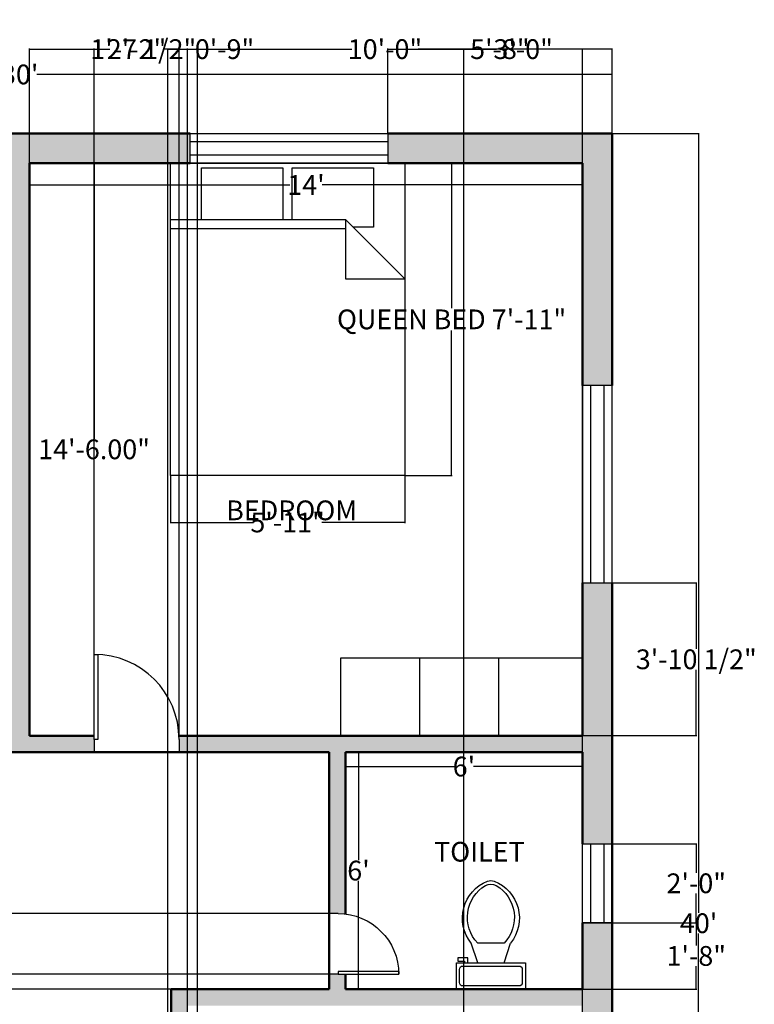
# Model space of a CAD drawing. Units: inches. Extents: x -19 to 426, y -15 to 535.
# Tile 4 of 4: x 202 to 426, y 235 to 535. Entities that reach past the tile are written whole.
import ezdxf

# ---------------------------------------------------------------- set-up
doc = ezdxf.new("R2010")
doc.units = ezdxf.units.IN
doc.header["$MEASUREMENT"] = 0
for name, color, linetype, lineweight in [('A-ANNO-DIMS', 3, 'Continuous', 18), ('A-AREA-IDEN', 7, 'Continuous', 25), ('A-DOOR', 4, 'Continuous', 25), ('A-FLOR-CABN', 40, 'Continuous', 25), ('A-FLOR-FIXT', 8, 'Continuous', 25), ('A-FURN', 40, 'Continuous', 25), ('A-GLAZ', 40, 'Continuous', 25), ('A-WALL', 7, 'Continuous', 50), ('A-WALL-PATT', 5, 'Continuous', 13)]:
    doc.layers.add(name, color=color, linetype=linetype, lineweight=lineweight)
doc.styles.get("Standard").update_dxf_attribs({"font": 'arial.ttf'})
doc.dimstyles.get("Standard").update_dxf_attribs({"dimtxt": 6, "dimasz": 0.18, "dimexe": 0.18, "dimexo": 0.0625, "dimgap": 0.09, "dimtad": 0, "dimtih": 1, "dimtoh": 1, "dimzin": 0, "dimdsep": 46, "dimlunit": 3, "dimtxsty": 'Standard', "dimcen": 0.09, "dimadec": 0, "dimazin": 0, "dimtfac": 1, "dimtofl": 0, "dimtmove": 0, "dimatfit": 3, "dimfxl": 1, "dimtolj": 1, "dimtzin": 0, "dimarcsym": 0})

# ---------------------------------------------------------------- blocks, each defined once
blk = doc.blocks.new('*D2')
at = {"layer": 'A-ANNO-DIMS', "color": 0, "lineweight": -2, "transparency": 16777216}
for p, q in [((301.43, 311.94), (301.43, 307.44)), ((373.43, 311.94), (373.43, 307.44)), ((301.61, 307.62), (334.57, 307.62)), ((373.25, 307.62), (340.3, 307.62))]:
    blk.add_line(p, q, dxfattribs=at)
at = {"layer": 'A-ANNO-DIMS', "color": 0, "transparency": 16777216}
for points in [[(301.61, 307.65), (301.61, 307.59), (301.43, 307.62)], [(373.25, 307.65), (373.25, 307.59), (373.43, 307.62)]]:
    blk.add_solid(points, dxfattribs=at)
at = {"layer": 'Defpoints', "color": 0, "transparency": 16777216}
for p in [(301.43, 312.01), (373.43, 312.01), (373.43, 307.62)]:
    blk.add_point(p, dxfattribs=at)
at = {"layer": 'A-ANNO-DIMS', "color": 0, "transparency": 16777216, "insert": (337.43, 307.62), "char_height": 6, "attachment_point": 5}
blk.add_mtext("\\A1;6'", dxfattribs=at)
blk = doc.blocks.new('*D3')
at = {"layer": 'A-ANNO-DIMS', "color": 0, "lineweight": -2, "transparency": 16777216}
for p, q in [((301.49, 312.01), (305.56, 312.01)), ((305.38, 311.83), (305.38, 279.16)), ((305.38, 240.19), (305.38, 272.85)), ((301.49, 240.01), (305.56, 240.01))]:
    blk.add_line(p, q, dxfattribs=at)
at = {"layer": 'A-ANNO-DIMS', "color": 0, "transparency": 16777216}
for points in [[(305.35, 311.83), (305.41, 311.83), (305.38, 312.01)], [(305.35, 240.19), (305.41, 240.19), (305.38, 240.01)]]:
    blk.add_solid(points, dxfattribs=at)
at = {"layer": 'Defpoints', "color": 0, "transparency": 16777216}
for p in [(301.43, 312.01), (301.43, 240.01), (305.38, 240.01)]:
    blk.add_point(p, dxfattribs=at)
at = {"layer": 'A-ANNO-DIMS', "color": 0, "transparency": 16777216, "insert": (305.38, 276.01), "char_height": 6, "attachment_point": 5}
blk.add_mtext("\\A1;6'", dxfattribs=at)
blk = doc.blocks.new('*D4')
at = {"layer": 'A-ANNO-DIMS', "color": 0, "lineweight": -2, "transparency": 16777216}
for p, q in [((205.43, 490.94), (205.43, 484.15)), ((373.43, 490.94), (373.43, 484.15)), ((205.61, 484.33), (284.53, 484.33)), ((373.25, 484.33), (294.33, 484.33))]:
    blk.add_line(p, q, dxfattribs=at)
at = {"layer": 'A-ANNO-DIMS', "color": 0, "transparency": 16777216}
for points in [[(205.61, 484.36), (205.61, 484.3), (205.43, 484.33)], [(373.25, 484.36), (373.25, 484.3), (373.43, 484.33)]]:
    blk.add_solid(points, dxfattribs=at)
at = {"layer": 'Defpoints', "color": 0, "transparency": 16777216}
for p in [(205.43, 491.01), (373.43, 491.01), (373.43, 484.33)]:
    blk.add_point(p, dxfattribs=at)
at = {"layer": 'A-ANNO-DIMS', "color": 0, "transparency": 16777216, "insert": (289.43, 484.33), "char_height": 6, "attachment_point": 5}
blk.add_mtext("\\A1;14'", dxfattribs=at)
blk = doc.blocks.new('Bed - Queen')
for p, q in [((0, -80.00003), (0, 0)), ((0, 0), (59.99999, 0)), ((59.99999, 0), (59.99999, -80.00003)), ((7.99999, -1.2), (28.79998, -1.2)), ((7.99999, -14.4), (7.99999, -1.2)), ((28.79998, -1.2), (28.79998, -14.4)), ((31.19999, -1.2), (51.99999, -1.2)), ((31.19999, -14.4), (31.19999, -1.2)), ((51.99999, -1.2), (51.99999, -16.4)), ((0, -14.4), (44.8, -14.4)), ((59.99999, -29.6), (44.8, -14.4)), ((44.8, -14.4), (44.8, -29.6)), ((44.8, -16.8), (0, -16.8)), ((51.99999, -16.4), (46.79936, -16.4)), ((44.8, -29.6), (59.99999, -29.6)), ((59.99999, -80.00003), (0, -80.00003))]:
    blk.add_line(p, q)
blk = doc.blocks.new('*U9')
for p, q in [((0, 0), (0, -6)), ((40, 0), (40, -6))]:
    blk.add_line(p, q)
blk.add_lwpolyline([(0, 0), (0, 40), (1.75, 40), (1.75, 0)], close=True)
blk.add_arc((0, 0), 40, 0, 90)
blk = doc.blocks.new('*U7')
for p, q in [((9.5, -6), (9.5, -2)), ((-10, -8.5), (-8, -8.5)), ((-10, -9.5), (-10, -8.5)), ((-8, -8.5), (-8, -8)), ((-7, -8), (-7, -9.5)), ((-4, -8), (-6, -14)), ((4, -8), (6, -14)), ((-7, -9.5), (-10, -9.5)), ((4, -14), (-4, -14))]:
    blk.add_line(p, q)
blk.add_lwpolyline([(10.5, -8), (10.5, 0), (-10.5, 0), (-10.5, -8)], close=True)
for points in [[(-9.5, -2), (-9.5, -6)], [(8.5, -1), (-8.5, -1)], [(-8.5, -7), (8.5, -7)]]:
    blk.add_lwpolyline(points)
for centre, radius, start, end in [((-8.62, -1.88), 0.884, 81.8699, 188.1301), ((8.62, -1.88), 0.884, 351.8699, 98.1301), ((-8.62, -6.12), 0.884, 171.8699, 278.1301), ((8.62, -6.12), 0.884, 261.8699, 8.1301), ((3.52, -21.58), 12.17, 141.4691, 247.9714), ((4.2, -21.82), 11.33, 136.3677, 238.9468), ((-3.52, -21.58), 12.17, 292.0284, 38.5307), ((-4.2, -21.82), 11.33, 301.053, 43.6321), ((0, -27.88), 4, 245.7318, 294.2682), ((0, -29), 4, 254.8605, 285.1395)]:
    blk.add_arc(centre, radius, start, end)
blk = doc.blocks.new('*D15')
at = {"layer": 'A-ANNO-DIMS', "color": 0, "lineweight": -2, "transparency": 16777216}
for p, q in [((205.49, 491.01), (225.21, 491.01)), ((225.03, 490.83), (225.03, 407.16)), ((225.03, 317.19), (225.03, 400.85)), ((205.49, 317.01), (225.21, 317.01))]:
    blk.add_line(p, q, dxfattribs=at)
at = {"layer": 'A-ANNO-DIMS', "color": 0, "transparency": 16777216}
for points in [[(225, 490.83), (225.06, 490.83), (225.03, 491.01)], [(225, 317.19), (225.06, 317.19), (225.03, 317.01)]]:
    blk.add_solid(points, dxfattribs=at)
at = {"layer": 'Defpoints', "color": 0, "transparency": 16777216}
for p in [(205.43, 491.01), (205.43, 317.01), (225.03, 317.01)]:
    blk.add_point(p, dxfattribs=at)
at = {"layer": 'A-ANNO-DIMS', "color": 0, "transparency": 16777216, "insert": (225.03, 404.01), "char_height": 6, "attachment_point": 5}
blk.add_mtext('\\A1;14\'-6.00"', dxfattribs=at)
blk = doc.blocks.new('*D18')
at = {"layer": 'A-ANNO-DIMS', "color": 0, "lineweight": -2, "transparency": 16777216}
for p, q in [((22.43, 500.07), (22.43, 518.1)), ((22.61, 517.92), (197.25, 517.92)), ((382.25, 517.92), (207.61, 517.92)), ((382.43, 500.07), (382.43, 518.1))]:
    blk.add_line(p, q, dxfattribs=at)
at = {"layer": 'A-ANNO-DIMS', "color": 0, "transparency": 16777216}
for points in [[(22.61, 517.95), (22.61, 517.89), (22.43, 517.92)], [(382.25, 517.95), (382.25, 517.89), (382.43, 517.92)]]:
    blk.add_solid(points, dxfattribs=at)
at = {"layer": 'Defpoints', "color": 0, "transparency": 16777216}
for p in [(382.43, 517.92), (22.43, 500.01), (382.43, 500.01)]:
    blk.add_point(p, dxfattribs=at)
at = {"layer": 'A-ANNO-DIMS', "color": 0, "transparency": 16777216, "insert": (202.43, 517.92), "char_height": 6, "attachment_point": 5}
blk.add_mtext("\\A1;30'", dxfattribs=at)
blk = doc.blocks.new('*D19')
at = {"layer": 'A-ANNO-DIMS', "color": 0, "lineweight": -2, "transparency": 16777216}
for p, q in [((382.49, 500.01), (408.92, 500.01)), ((408.74, 499.83), (408.74, 263.16)), ((408.74, 20.19), (408.74, 256.85)), ((382.49, 20.01), (408.92, 20.01))]:
    blk.add_line(p, q, dxfattribs=at)
at = {"layer": 'A-ANNO-DIMS', "color": 0, "transparency": 16777216}
for points in [[(408.71, 499.83), (408.77, 499.83), (408.74, 500.01)], [(408.71, 20.19), (408.77, 20.19), (408.74, 20.01)]]:
    blk.add_solid(points, dxfattribs=at)
at = {"layer": 'Defpoints', "color": 0, "transparency": 16777216}
for p in [(382.43, 500.01), (382.43, 20.01), (408.74, 20.01)]:
    blk.add_point(p, dxfattribs=at)
at = {"layer": 'A-ANNO-DIMS', "color": 0, "transparency": 16777216, "insert": (408.74, 260.01), "char_height": 6, "attachment_point": 5}
blk.add_mtext("\\A1;40'", dxfattribs=at)
blk = doc.blocks.new('WIN-60IN')
for p, q in [((0, 6.5), (60, 6.5)), ((0, 2.5), (60, 2.5))]:
    blk.add_line(p, q)
blk.add_lwpolyline([(0, 9), (60, 9), (60, 0), (0, 0)], close=True)
blk = doc.blocks.new('*D24')
at = {"layer": 'A-ANNO-DIMS', "color": 0, "lineweight": -2, "transparency": 16777216}
for p, q in [((319.5, 490.97), (333.86, 490.97)), ((333.68, 490.79), (333.68, 446.87)), ((333.68, 396.21), (333.68, 440.12)), ((319.5, 396.03), (333.86, 396.03))]:
    blk.add_line(p, q, dxfattribs=at)
at = {"layer": 'A-ANNO-DIMS', "color": 0, "transparency": 16777216}
for points in [[(333.65, 490.79), (333.71, 490.79), (333.68, 490.97)], [(333.65, 396.21), (333.71, 396.21), (333.68, 396.03)]]:
    blk.add_solid(points, dxfattribs=at)
at = {"layer": 'Defpoints', "color": 0, "transparency": 16777216}
for p in [(319.44, 490.97), (333.68, 490.97), (319.44, 396.03)]:
    blk.add_point(p, dxfattribs=at)
at = {"layer": 'A-ANNO-DIMS', "color": 0, "transparency": 16777216, "insert": (333.68, 443.5), "char_height": 6, "attachment_point": 5}
blk.add_mtext('\\A1;QUEEN BED 7\'-11"', dxfattribs=at)
blk = doc.blocks.new('*D25')
at = {"layer": 'A-ANNO-DIMS', "color": 0, "lineweight": -2, "transparency": 16777216}
for p, q in [((248.23, 395.97), (248.23, 381.61)), ((319.44, 395.97), (319.44, 381.61)), ((248.41, 381.79), (273.44, 381.79)), ((319.26, 381.79), (294.23, 381.79))]:
    blk.add_line(p, q, dxfattribs=at)
at = {"layer": 'A-ANNO-DIMS', "color": 0, "transparency": 16777216}
for points in [[(248.41, 381.82), (248.41, 381.76), (248.23, 381.79)], [(319.26, 381.82), (319.26, 381.76), (319.44, 381.79)]]:
    blk.add_solid(points, dxfattribs=at)
at = {"layer": 'Defpoints', "color": 0, "transparency": 16777216}
for p in [(248.23, 396.03), (319.44, 396.03), (319.44, 381.79)]:
    blk.add_point(p, dxfattribs=at)
at = {"layer": 'A-ANNO-DIMS', "color": 0, "transparency": 16777216, "insert": (283.84, 381.79), "char_height": 6, "attachment_point": 5}
blk.add_mtext('\\A1;5\'-11"', dxfattribs=at)
blk = doc.blocks.new('*D32')
at = {"layer": 'A-ANNO-DIMS', "color": 0, "lineweight": -2, "transparency": 16777216}
for p, q in [((253.43, 115.07), (253.43, 525.79)), ((253.61, 525.61), (303.32, 525.61)), ((373.25, 525.61), (323.55, 525.61)), ((373.43, 115.07), (373.43, 525.79))]:
    blk.add_line(p, q, dxfattribs=at)
at = {"layer": 'A-ANNO-DIMS', "color": 0, "transparency": 16777216}
for points in [[(253.61, 525.64), (253.61, 525.58), (253.43, 525.61)], [(373.25, 525.64), (373.25, 525.58), (373.43, 525.61)]]:
    blk.add_solid(points, dxfattribs=at)
at = {"layer": 'Defpoints', "color": 0, "transparency": 16777216}
for p in [(373.43, 525.61), (253.43, 115.01), (373.43, 115.01)]:
    blk.add_point(p, dxfattribs=at)
at = {"layer": 'A-ANNO-DIMS', "color": 0, "transparency": 16777216, "insert": (313.43, 525.61), "char_height": 6, "attachment_point": 5}
blk.add_mtext('\\A1;10\'-0"', dxfattribs=at)
blk = doc.blocks.new('*D37')
at = {"layer": 'A-ANNO-DIMS', "color": 0, "lineweight": -2, "transparency": 16777216}
for p, q in [((314.27, 500.07), (314.27, 525.79)), ((314.45, 525.61), (340.29, 525.61)), ((382.25, 525.61), (356.42, 525.61)), ((382.43, 500.07), (382.43, 525.79))]:
    blk.add_line(p, q, dxfattribs=at)
at = {"layer": 'A-ANNO-DIMS', "color": 0, "transparency": 16777216}
for points in [[(314.45, 525.64), (314.45, 525.58), (314.27, 525.61)], [(382.25, 525.64), (382.25, 525.58), (382.43, 525.61)]]:
    blk.add_solid(points, dxfattribs=at)
at = {"layer": 'Defpoints', "color": 0, "transparency": 16777216}
for p in [(382.43, 525.61), (314.27, 500.01), (382.43, 500.01)]:
    blk.add_point(p, dxfattribs=at)
at = {"layer": 'A-ANNO-DIMS', "color": 0, "transparency": 16777216, "insert": (348.35, 525.61), "char_height": 6, "attachment_point": 5}
blk.add_mtext('\\A1;5\'-8"', dxfattribs=at)
blk = doc.blocks.new('*D48')
at = {"layer": 'A-ANNO-DIMS', "color": 0, "lineweight": -2, "transparency": 16777216}
for p, q in [((373.49, 260.15), (408.21, 260.15)), ((408.03, 259.97), (408.03, 253.23)), ((408.03, 240.19), (408.03, 246.93)), ((373.49, 240.01), (408.21, 240.01))]:
    blk.add_line(p, q, dxfattribs=at)
at = {"layer": 'A-ANNO-DIMS', "color": 0, "transparency": 16777216}
for points in [[(408, 259.97), (408.06, 259.97), (408.03, 260.15)], [(408, 240.19), (408.06, 240.19), (408.03, 240.01)]]:
    blk.add_solid(points, dxfattribs=at)
at = {"layer": 'Defpoints', "color": 0, "transparency": 16777216}
for p in [(373.43, 260.15), (408.03, 260.15), (373.43, 240.01)]:
    blk.add_point(p, dxfattribs=at)
at = {"layer": 'A-ANNO-DIMS', "color": 0, "transparency": 16777216, "insert": (408.03, 250.08), "char_height": 6, "attachment_point": 5}
blk.add_mtext('\\A1;1\'-8"', dxfattribs=at)
blk = doc.blocks.new('*D49')
at = {"layer": 'A-ANNO-DIMS', "color": 0, "lineweight": -2, "transparency": 16777216}
for p, q in [((373.49, 284.15), (408.21, 284.15)), ((408.03, 283.97), (408.03, 275.3)), ((408.03, 260.33), (408.03, 269)), ((373.49, 260.15), (408.21, 260.15))]:
    blk.add_line(p, q, dxfattribs=at)
at = {"layer": 'A-ANNO-DIMS', "color": 0, "transparency": 16777216}
for points in [[(408, 283.97), (408.06, 283.97), (408.03, 284.15)], [(408, 260.33), (408.06, 260.33), (408.03, 260.15)]]:
    blk.add_solid(points, dxfattribs=at)
at = {"layer": 'Defpoints', "color": 0, "transparency": 16777216}
for p in [(373.43, 284.15), (408.03, 284.15), (373.43, 260.15)]:
    blk.add_point(p, dxfattribs=at)
at = {"layer": 'A-ANNO-DIMS', "color": 0, "transparency": 16777216, "insert": (408.03, 272.15), "char_height": 6, "attachment_point": 5}
blk.add_mtext('\\A1;2\'-0"', dxfattribs=at)
blk = doc.blocks.new('*D50')
at = {"layer": 'A-ANNO-DIMS', "color": 0, "lineweight": -2, "transparency": 16777216}
for p, q in [((373.49, 363.41), (408.21, 363.41)), ((408.03, 363.23), (408.03, 343.4)), ((408.03, 317.19), (408.03, 337.01)), ((373.49, 317.01), (408.21, 317.01))]:
    blk.add_line(p, q, dxfattribs=at)
at = {"layer": 'A-ANNO-DIMS', "color": 0, "transparency": 16777216}
for points in [[(408, 363.23), (408.06, 363.23), (408.03, 363.41)], [(408, 317.19), (408.06, 317.19), (408.03, 317.01)]]:
    blk.add_solid(points, dxfattribs=at)
at = {"layer": 'Defpoints', "color": 0, "transparency": 16777216}
for p in [(373.43, 363.41), (408.03, 363.41), (373.43, 317.01)]:
    blk.add_point(p, dxfattribs=at)
at = {"layer": 'A-ANNO-DIMS', "color": 0, "transparency": 16777216, "insert": (408.03, 340.21), "char_height": 6, "attachment_point": 5}
blk.add_mtext('\\A1;3\'-10 1/2"', dxfattribs=at)
blk = doc.blocks.new('*D53')
at = {"layer": 'A-ANNO-DIMS', "color": 0, "lineweight": -2, "transparency": 16777216}
for p, q in [((205.43, 317.07), (205.43, 525.79)), ((205.61, 525.61), (224.85, 525.61)), ((225.03, 317.07), (225.03, 525.79)), ((225.03, 525.61), (225.21, 525.61))]:
    blk.add_line(p, q, dxfattribs=at)
at = {"layer": 'A-ANNO-DIMS', "color": 0, "transparency": 16777216}
for points in [[(205.61, 525.64), (205.61, 525.58), (205.43, 525.61)], [(224.85, 525.64), (224.85, 525.58), (225.03, 525.61)]]:
    blk.add_solid(points, dxfattribs=at)
at = {"layer": 'Defpoints', "color": 0, "transparency": 16777216}
for p in [(225.03, 525.61), (205.43, 317.01), (225.03, 317.01)]:
    blk.add_point(p, dxfattribs=at)
at = {"layer": 'A-ANNO-DIMS', "color": 0, "transparency": 16777216, "insert": (239.99, 525.61), "char_height": 6, "attachment_point": 5}
blk.add_mtext('\\A1;1\'-7 1/2"', dxfattribs=at)
blk = doc.blocks.new('*D54')
at = {"layer": 'A-ANNO-DIMS', "color": 0, "lineweight": -2, "transparency": 16777216}
for p, q in [((225.03, 317.07), (225.03, 525.79)), ((225.21, 525.61), (229.82, 525.61)), ((250.67, 525.61), (246.06, 525.61)), ((250.85, 317.07), (250.85, 525.79))]:
    blk.add_line(p, q, dxfattribs=at)
at = {"layer": 'A-ANNO-DIMS', "color": 0, "transparency": 16777216}
for points in [[(225.21, 525.64), (225.21, 525.58), (225.03, 525.61)], [(250.67, 525.64), (250.67, 525.58), (250.85, 525.61)]]:
    blk.add_solid(points, dxfattribs=at)
at = {"layer": 'Defpoints', "color": 0, "transparency": 16777216}
for p in [(250.85, 525.61), (225.03, 317.01), (250.85, 317.01)]:
    blk.add_point(p, dxfattribs=at)
at = {"layer": 'A-ANNO-DIMS', "color": 0, "transparency": 16777216, "insert": (237.94, 525.61), "char_height": 6, "attachment_point": 5}
blk.add_mtext('\\A1;2\'-2"', dxfattribs=at)
blk = doc.blocks.new('*D55')
at = {"layer": 'A-ANNO-DIMS', "color": 0, "lineweight": -2, "transparency": 16777216}
for p, q in [((296.37, 244.52), (-3.35, 244.52)), ((-3.17, 244.52), (-3.17, 244.7)), ((-3.17, 244.7), (-2.99, 244.7)), ((-3.17, 240.19), (-3.17, 244.34)), ((296.37, 240.01), (-3.35, 240.01))]:
    blk.add_line(p, q, dxfattribs=at)
at = {"layer": 'A-ANNO-DIMS', "color": 0, "transparency": 16777216}
for points in [[(-3.2, 244.34), (-3.14, 244.34), (-3.17, 244.52)], [(-3.2, 240.19), (-3.14, 240.19), (-3.17, 240.01)]]:
    blk.add_solid(points, dxfattribs=at)
at = {"layer": 'Defpoints', "color": 0, "transparency": 16777216}
for p in [(-3.17, 244.52), (296.43, 244.52), (296.43, 240.01)]:
    blk.add_point(p, dxfattribs=at)
at = {"layer": 'A-ANNO-DIMS', "color": 0, "transparency": 16777216, "insert": (12.07, 244.7), "char_height": 6, "attachment_point": 5}
blk.add_mtext('\\A1;0\'-4 1/2"', dxfattribs=at)
blk = doc.blocks.new('*D56')
at = {"layer": 'A-ANNO-DIMS', "color": 0, "lineweight": -2, "transparency": 16777216}
for p, q in [((296.37, 262.94), (-3.35, 262.94)), ((-3.17, 262.76), (-3.17, 256.93)), ((-3.17, 244.7), (-3.17, 250.54)), ((296.37, 244.52), (-3.35, 244.52))]:
    blk.add_line(p, q, dxfattribs=at)
at = {"layer": 'A-ANNO-DIMS', "color": 0, "transparency": 16777216}
for points in [[(-3.2, 262.76), (-3.14, 262.76), (-3.17, 262.94)], [(-3.2, 244.7), (-3.14, 244.7), (-3.17, 244.52)]]:
    blk.add_solid(points, dxfattribs=at)
at = {"layer": 'Defpoints', "color": 0, "transparency": 16777216}
for p in [(-3.17, 262.94), (296.43, 262.94), (296.43, 244.52)]:
    blk.add_point(p, dxfattribs=at)
at = {"layer": 'A-ANNO-DIMS', "color": 0, "transparency": 16777216, "insert": (-3.17, 253.73), "char_height": 6, "attachment_point": 5}
blk.add_mtext('\\A1;1\'-6 1/2"', dxfattribs=at)
blk = doc.blocks.new('*D61')
at = {"layer": 'A-ANNO-DIMS', "color": 0, "lineweight": -2, "transparency": 16777216}
for p, q in [((247.43, 29.07), (247.43, 525.79)), ((247.61, 525.61), (256.25, 525.61)), ((256.43, 29.07), (256.43, 525.79)), ((256.43, 525.61), (256.61, 525.61))]:
    blk.add_line(p, q, dxfattribs=at)
at = {"layer": 'A-ANNO-DIMS', "color": 0, "transparency": 16777216}
for points in [[(247.61, 525.64), (247.61, 525.58), (247.43, 525.61)], [(256.25, 525.64), (256.25, 525.58), (256.43, 525.61)]]:
    blk.add_solid(points, dxfattribs=at)
at = {"layer": 'Defpoints', "color": 0, "transparency": 16777216}
for p in [(256.43, 525.61), (247.43, 29.01), (256.43, 29.01)]:
    blk.add_point(p, dxfattribs=at)
at = {"layer": 'A-ANNO-DIMS', "color": 0, "transparency": 16777216, "insert": (264.68, 525.61), "char_height": 6, "attachment_point": 5}
blk.add_mtext('\\A1;0\'-9"', dxfattribs=at)
blk = doc.blocks.new('*D62')
at = {"layer": 'A-ANNO-DIMS', "color": 0, "lineweight": -2, "transparency": 16777216}
for p, q in [((337.43, 29.07), (337.43, 525.79)), ((337.61, 525.61), (347.37, 525.61)), ((373.25, 525.61), (363.5, 525.61)), ((373.43, 29.07), (373.43, 525.79))]:
    blk.add_line(p, q, dxfattribs=at)
at = {"layer": 'A-ANNO-DIMS', "color": 0, "transparency": 16777216}
for points in [[(337.61, 525.64), (337.61, 525.58), (337.43, 525.61)], [(373.25, 525.64), (373.25, 525.58), (373.43, 525.61)]]:
    blk.add_solid(points, dxfattribs=at)
at = {"layer": 'Defpoints', "color": 0, "transparency": 16777216}
for p in [(373.43, 525.61), (337.43, 29.01), (373.43, 29.01)]:
    blk.add_point(p, dxfattribs=at)
at = {"layer": 'A-ANNO-DIMS', "color": 0, "transparency": 16777216, "insert": (355.43, 525.61), "char_height": 6, "attachment_point": 5}
blk.add_mtext('\\A1;3\'-0"', dxfattribs=at)

msp = doc.modelspace()

# ---------------------------------------------------------------- hatches: boundary and pattern name
at = {"layer": 'A-WALL-PATT'}
h = msp.add_hatch(color=256, dxfattribs=at)
h.dxf.hatch_style = 1
h.paths.add_polyline_path([(205.432, 491.007), (254.275, 491.007), (254.275, 500.007), (22.432, 500.007), (22.432, 449.048), (31.432, 449.048), (31.432, 491.007), (199.432, 491.007), (199.432, 312.007), (225.033, 312.007), (225.033, 315.882), (225.033, 317.007), (205.432, 317.007)])
h.paths.add_polyline_path([(382.432, 500.007), (314.275, 500.007), (314.275, 491.007), (373.432, 491.007), (373.432, 423.411), (382.432, 423.411)])
h.paths.add_polyline_path([(382.432, 363.411), (373.432, 363.411), (373.432, 317.007), (250.847, 317.007, -0.0108825), (250.871, 315.882), (250.871, 312.007), (296.432, 312.007), (296.432, 262.945), (299.196, 262.945, -0.0304399), (301.432, 262.809), (301.432, 312.007), (373.432, 312.007), (373.432, 284.151), (382.432, 284.151)])
h = msp.add_hatch(color=256, dxfattribs=at)
h.dxf.hatch_style = 1
h.paths.add_polyline_path([(253.432, 235.007), (373.432, 235.007), (373.432, 196.661), (382.432, 196.661), (382.432, 260.151), (373.432, 260.151), (373.432, 240.007), (356.117, 240.007), (356.117, 239.974), (335.117, 239.974), (301.432, 240.007), (301.432, 244.523), (299.196, 244.523), (296.432, 244.523), (296.432, 240.007), (248.432, 240.007), (248.432, 153.518), (253.083, 153.518, -0.0028192), (253.432, 153.516)])

# ---------------------------------------------------------------- linework, layer by layer
at = {"layer": 'A-FLOR-CABN'}
for p, q in [((300.013, 317.007), (300.013, 340.611)), ((300.013, 340.611), (373.432, 340.611)), ((324.013, 317.007), (324.013, 340.611)), ((348.013, 317.007), (348.013, 340.611))]:
    msp.add_line(p, q, dxfattribs=at)
at = {"layer": 'A-GLAZ'}
for p, q in [((375.932, 284.151), (375.932, 260.151)), ((379.932, 284.151), (379.932, 260.151))]:
    msp.add_line(p, q, dxfattribs=at)
msp.add_lwpolyline([(373.432, 284.151), (382.432, 284.151), (382.432, 260.151), (373.432, 260.151)], close=True, dxfattribs=at)
at = {"layer": 'A-WALL'}
for points in [[(254.275, 500.007), (22.432, 500.007), (22.432, 448.979)], [(382.432, 423.411), (382.432, 500.007), (314.275, 500.007)], [(205.432, 317.007), (205.432, 491.007)], [(254.275, 491.007), (205.432, 491.007)], [(373.432, 491.007), (314.275, 491.007)], [(373.432, 423.411), (373.432, 491.007)], [(373.432, 317.007), (373.432, 363.411)], [(382.432, 284.151), (382.432, 363.411)], [(225.033, 317.007), (205.432, 317.007)], [(373.432, 317.007), (250.847, 317.007)], [(296.432, 312.007), (199.432, 312.007)], [(296.432, 240.007), (296.432, 312.007)], [(373.432, 312.007), (301.432, 312.007)], [(301.432, 262.809), (301.432, 312.007)], [(373.432, 284.151), (373.432, 312.007)], [(382.432, 196.661), (382.432, 284.151)], [(373.432, 240.007), (373.432, 260.151)], [(301.432, 240.007), (301.432, 244.523)], [(248.432, 115.007), (248.432, 240.007)], [(296.432, 240.007), (248.432, 240.007)], [(373.432, 240.007), (301.432, 240.007)]]:
    msp.add_lwpolyline(points, dxfattribs=at)

# ---------------------------------------------------------------- block references
at = {"layer": 'A-DOOR', "xscale": 0.6459463181604524, "yscale": 0.6459463181604524, "zscale": 0.6459463181604524}
msp.add_blockref('*U9', (225.033, 315.882), dxfattribs=at)
at = {"layer": 'A-DOOR', "xscale": -0.4605382083706444, "yscale": 0.4605382083706444, "zscale": 0.4605382083706444, "rotation": 270}
msp.add_blockref('*U9', (299.196, 244.523), dxfattribs=at)
at = {"layer": 'A-FLOR-FIXT', "xscale": -1, "rotation": 180}
msp.add_blockref('*U7', (345.617, 239.974), dxfattribs=at)
at = {"layer": 'A-FURN', "xscale": 1.186711706459686, "yscale": 1.186711706459686, "zscale": 1.186711706459686}
msp.add_blockref('Bed - Queen', (248.235, 490.965), dxfattribs=at)
at = {"layer": 'A-GLAZ'}
msp.add_blockref('WIN-60IN', (254.275, 491.007), dxfattribs=at)
at = {"layer": 'A-GLAZ', "extrusion": (0, 0, -1), "zscale": -1, "rotation": 269.9999999999999}
msp.add_blockref('WIN-60IN', (-382.432, 423.411), dxfattribs=at)

# ---------------------------------------------------------------- texts
at = {"layer": 'A-AREA-IDEN', "char_height": 6, "attachment_point": 1}
for s, insert in [('{BEDROOM}', (265.16, 388.469)), ('{TOILET}', (328.348, 284.743))]:
    msp.add_mtext_dynamic_manual_height_columns(s, width=105.43776, gutter_width=1, heights=[0.207], dxfattribs=dict(at, insert=insert))

# ---------------------------------------------------------------- dimensions: what is measured, and where the dimension line sits
at = {"layer": 'A-ANNO-DIMS'}
for base, p1, p2, override, picture, middle in [((225.033, 525.607), (205.432, 317.007), (225.033, 317.007), {"dimdec": 1, "dimlfac": 1, "dimrnd": 0, "dimzin": 1, "dimdsep": 46, "dimlunit": 4, "dimfrac": 2}, '*D53', (239.986, 525.607)), ((250.847, 525.607), (225.033, 317.007), (250.847, 317.007), {"dimdec": 1, "dimlfac": 1, "dimrnd": 0, "dimzin": 1, "dimdsep": 46, "dimlunit": 4, "dimfrac": 2}, '*D54', (237.94, 525.607)), ((256.432, 525.607), (247.432, 29.007), (256.432, 29.007), {"dimdec": 1, "dimlfac": 1, "dimrnd": 0, "dimzin": 1, "dimdsep": 46, "dimlunit": 4, "dimfrac": 2}, '*D61', (264.677, 525.607)), ((373.432, 525.607), (253.432, 115.007), (373.432, 115.007), {"dimdec": 1, "dimlfac": 1, "dimrnd": 0, "dimzin": 1, "dimdsep": 46, "dimlunit": 4, "dimfrac": 2}, '*D32', (313.432, 525.607)), ((382.432, 525.607), (314.275, 500.007), (382.432, 500.007), {"dimdec": 1, "dimlfac": 1, "dimrnd": 0, "dimzin": 1, "dimdsep": 46, "dimlunit": 4, "dimfrac": 2}, '*D37', (348.354, 525.607)), ((373.432, 525.607), (337.432, 29.007), (373.432, 29.007), {"dimdec": 1, "dimlfac": 1, "dimrnd": 0, "dimzin": 1, "dimdsep": 46, "dimlunit": 4, "dimfrac": 2}, '*D62', (355.432, 525.607)), ((382.432, 517.915), (22.432, 500.007), (382.432, 500.007), {"dimclrd": 0, "dimclre": 0, "dimclrt": 0}, '*D18', (202.432, 517.915)), ((373.432, 484.332), (205.432, 491.007), (373.432, 491.007), {"dimclrd": 0, "dimclre": 0, "dimclrt": 0}, '*D4', (289.432, 484.332)), ((319.438, 381.788), (248.235, 396.028), (319.438, 396.028), {"dimdec": 1, "dimlfac": 1, "dimrnd": 0, "dimzin": 1, "dimdsep": 46, "dimlunit": 4, "dimfrac": 2}, '*D25', (283.836, 381.788)), ((373.432, 307.622), (301.432, 312.007), (373.432, 312.007), {"dimclrd": 0, "dimclre": 0, "dimclrt": 0}, '*D2', (337.432, 307.622))]:
    dim = msp.add_linear_dim(base=base, p1=p1, p2=p2, dimstyle='Standard', override=override, dxfattribs=at)
    dim.commit()
    dim.dimension.update_dxf_attribs({"geometry": picture, "text_midpoint": middle})
for base, p1, p2, override, picture, middle in [((408.736, 20.007), (382.432, 500.007), (382.432, 20.007), {"dimclrd": 0, "dimclre": 0, "dimclrt": 0}, '*D19', (408.736, 260.007)), ((225.033, 317.007), (205.432, 491.007), (205.432, 317.007), {"dimclrd": 0, "dimclre": 0, "dimclrt": 0}, '*D15', (225.033, 404.007)), ((408.032, 363.411), (373.432, 317.007), (373.432, 363.411), {"dimdec": 1, "dimlfac": 1, "dimrnd": 0, "dimzin": 1, "dimdsep": 46, "dimlunit": 4, "dimfrac": 2}, '*D50', (408.032, 340.209)), ((305.38, 240.007), (301.432, 312.007), (301.432, 240.007), {"dimclrd": 0, "dimclre": 0, "dimclrt": 0}, '*D3', (305.38, 276.007)), ((408.032, 284.151), (373.432, 260.151), (373.432, 284.151), {"dimdec": 1, "dimlfac": 1, "dimrnd": 0, "dimzin": 1, "dimdsep": 46, "dimlunit": 4, "dimfrac": 2}, '*D49', (408.032, 272.151)), ((-3.168, 262.945), (296.432, 244.523), (296.432, 262.945), {"dimdec": 1, "dimlfac": 1, "dimrnd": 0, "dimzin": 1, "dimdsep": 46, "dimlunit": 4, "dimfrac": 2}, '*D56', (-3.168, 253.734)), ((408.032, 260.151), (373.432, 240.007), (373.432, 260.151), {"dimdec": 1, "dimlfac": 1, "dimrnd": 0, "dimzin": 1, "dimdsep": 46, "dimlunit": 4, "dimfrac": 2}, '*D48', (408.032, 250.079)), ((-3.168, 244.523), (296.432, 240.007), (296.432, 244.523), {"dimdec": 1, "dimlfac": 1, "dimrnd": 0, "dimzin": 1, "dimdsep": 46, "dimlunit": 4, "dimfrac": 2}, '*D55', (12.068, 244.703))]:
    dim = msp.add_linear_dim(base=base, p1=p1, p2=p2, angle=90, dimstyle='Standard', override=override, dxfattribs=at)
    dim.commit()
    dim.dimension.update_dxf_attribs({"geometry": picture, "text_midpoint": middle})
dim = msp.add_linear_dim(base=(333.678, 490.965), p1=(319.438, 396.028), p2=(319.438, 490.965), angle=90, text='QUEEN BED <>', dimstyle='Standard', override={"dimdec": 1, "dimlfac": 1, "dimrnd": 0, "dimzin": 1, "dimdsep": 46, "dimlunit": 4, "dimfrac": 2}, dxfattribs=at)
dim.commit()
dim.dimension.update_dxf_attribs({"geometry": '*D24', "text_midpoint": (333.678, 443.497)})

doc.saveas('drawing.dxf')
